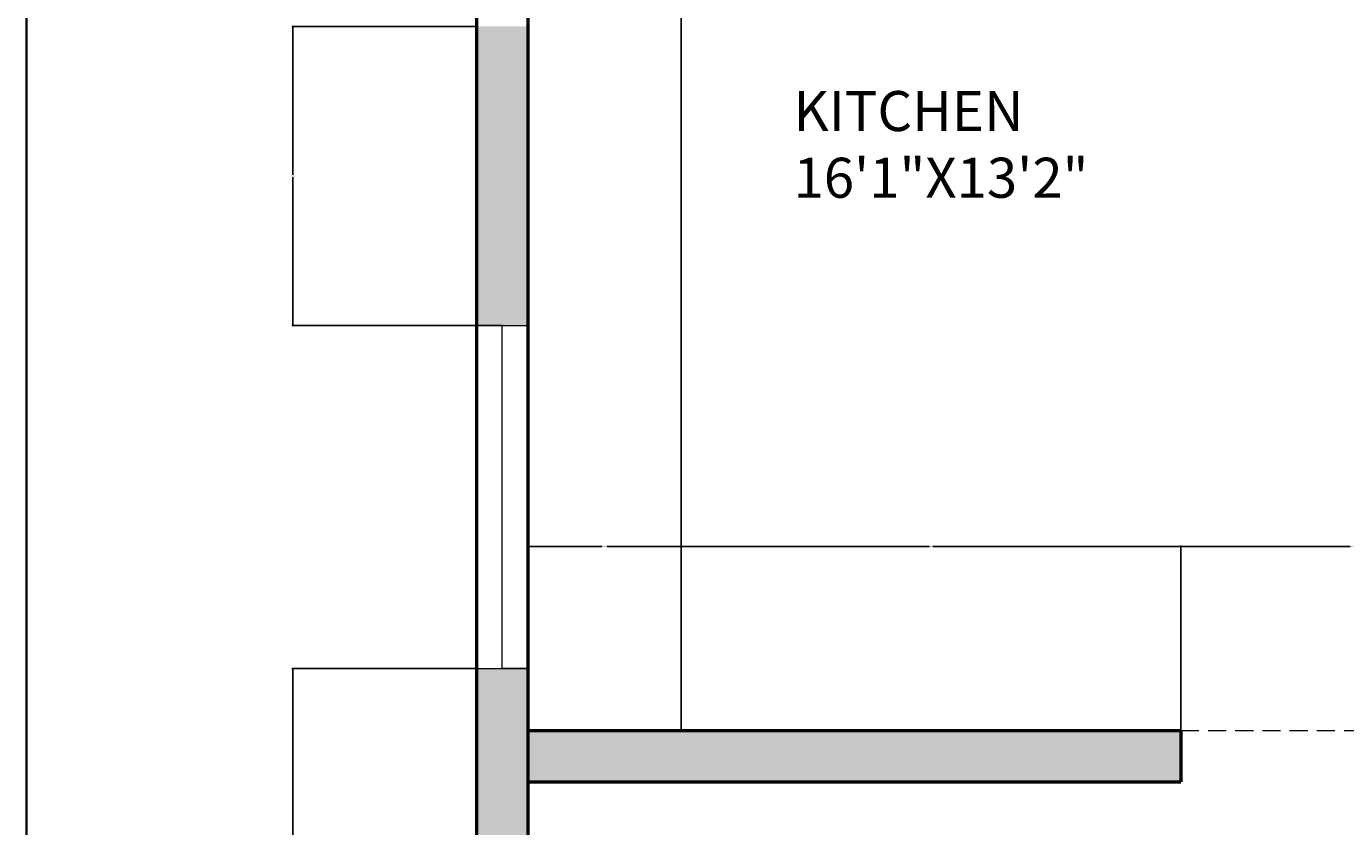
# Model space of a CAD drawing. Units: inches. Extents: x 1676 to 2199, y 1657 to 2783.
# Tile 5 of 10: x 1676 to 1907, y 2066 to 2206. Entities that reach past the tile are written whole.
import ezdxf

# ---------------------------------------------------------------- set-up
doc = ezdxf.new("R2010")
doc.units = ezdxf.units.IN
doc.linetypes.add('HIDDEN2', pattern=[4.7625, 3.175, -1.5875])
for name, color, linetype, lineweight in [('A-ANNO-DIMS', 2, 'Continuous', 18), ('A-ANNO-TTLB', 7, 'Continuous', 35), ('A-AREA-IDEN', 7, 'Continuous', 18), ('A-FLOR-CASE', 7, 'Continuous', 25), ('A-GLAZ', 4, 'Continuous', 18), ('A-WALL', 7, 'Continuous', 50), ('A-WALL-HIDN', 253, 'HIDDEN2', 18)]:
    doc.layers.add(name, color=color, linetype=linetype, lineweight=lineweight)
doc.layers.add('A-WALL-PATT', color=251, linetype='Continuous', lineweight=13, true_color=0x636466)
doc.styles.get("Standard").update_dxf_attribs({"font": 'arial.ttf'})
doc.dimstyles.get("Standard").update_dxf_attribs({"dimtxt": 0.18, "dimasz": 0.18, "dimexe": 0.18, "dimexo": 0.0625, "dimgap": 0.09, "dimtad": 0, "dimtih": 1, "dimtoh": 1, "dimdec": 4, "dimzin": 0, "dimdsep": 46, "dimtxsty": 'Standard', "dimcen": 0.09, "dimadec": 0, "dimazin": 0, "dimtfac": 1, "dimtdec": 4, "dimtofl": 0, "dimtmove": 0, "dimatfit": 3, "dimfxl": 1, "dimtolj": 1, "dimtzin": 0, "dimarcsym": 0})

# ---------------------------------------------------------------- blocks, each defined once
blk = doc.blocks.new('WIN-60')
for p, q in [((0, 0), (9, 0)), ((9, 0), (4.5, 0)), ((4.5, 0), (4.5, -60)), ((4.5, -60), (0, -60)), ((0, -60), (9, -60))]:
    blk.add_line(p, q)
blk = doc.blocks.new('*D26')
at = {"layer": 'A-ANNO-DIMS', "color": 0, "lineweight": -2, "transparency": 16777216}
for p, q in [((1755.01, 2093.92), (1722.74, 2093.92)), ((1722.92, 2093.74), (1722.92, 2056.93)), ((1722.92, 2019.75), (1722.92, 2056.56)), ((1755.01, 2019.57), (1722.74, 2019.57))]:
    blk.add_line(p, q, dxfattribs=at)
at = {"layer": 'A-ANNO-DIMS', "color": 0, "transparency": 16777216}
for points in [[(1722.89, 2093.74), (1722.95, 2093.74), (1722.92, 2093.92)], [(1722.89, 2019.75), (1722.95, 2019.75), (1722.92, 2019.57)]]:
    blk.add_solid(points, dxfattribs=at)
at = {"layer": 'Defpoints', "color": 0, "transparency": 16777216}
for p in [(1722.92, 2093.92), (1755.07, 2093.92), (1755.07, 2019.57)]:
    blk.add_point(p, dxfattribs=at)
at = {"layer": 'A-ANNO-DIMS', "color": 0, "transparency": 16777216, "insert": (1722.92, 2056.75), "char_height": 0.18, "attachment_point": 5}
blk.add_mtext('\\A1;74.35', dxfattribs=at)
blk = doc.blocks.new('*D27')
at = {"layer": 'A-ANNO-DIMS', "color": 0, "lineweight": -2, "transparency": 16777216}
for p, q in [((1755.01, 2206.26), (1722.74, 2206.26)), ((1722.92, 2206.08), (1722.92, 2180.27)), ((1722.92, 2154.1), (1722.92, 2179.91)), ((1755.01, 2153.92), (1722.74, 2153.92))]:
    blk.add_line(p, q, dxfattribs=at)
at = {"layer": 'A-ANNO-DIMS', "color": 0, "transparency": 16777216}
for points in [[(1722.89, 2206.08), (1722.95, 2206.08), (1722.92, 2206.26)], [(1722.89, 2154.1), (1722.95, 2154.1), (1722.92, 2153.92)]]:
    blk.add_solid(points, dxfattribs=at)
at = {"layer": 'Defpoints', "color": 0, "transparency": 16777216}
for p in [(1722.92, 2206.26), (1755.07, 2206.26), (1755.07, 2153.92)]:
    blk.add_point(p, dxfattribs=at)
at = {"layer": 'A-ANNO-DIMS', "color": 0, "transparency": 16777216, "insert": (1722.92, 2180.09), "char_height": 0.18, "attachment_point": 5}
blk.add_mtext('\\A1;52.34', dxfattribs=at)
blk = doc.blocks.new('*D49')
at = {"layer": 'A-ANNO-DIMS', "color": 0, "lineweight": -2, "transparency": 16777216}
for p, q in [((1878.39, 2083.15), (1878.39, 2115.42)), ((1878.57, 2115.24), (1908.02, 2115.24)), ((1938.22, 2115.24), (1908.78, 2115.24)), ((1938.4, 2083.15), (1938.4, 2115.42))]:
    blk.add_line(p, q, dxfattribs=at)
at = {"layer": 'A-ANNO-DIMS', "color": 0, "transparency": 16777216}
for points in [[(1878.57, 2115.27), (1878.57, 2115.21), (1878.39, 2115.24)], [(1938.22, 2115.27), (1938.22, 2115.21), (1938.4, 2115.24)]]:
    blk.add_solid(points, dxfattribs=at)
at = {"layer": 'Defpoints', "color": 0, "transparency": 16777216}
for p in [(1938.4, 2115.24), (1878.39, 2083.09), (1938.4, 2083.09)]:
    blk.add_point(p, dxfattribs=at)
at = {"layer": 'A-ANNO-DIMS', "color": 0, "transparency": 16777216, "insert": (1908.4, 2115.24), "char_height": 0.18, "attachment_point": 5}
blk.add_mtext('\\A1;60.01', dxfattribs=at)
blk = doc.blocks.new('*D50')
at = {"layer": 'A-ANNO-DIMS', "color": 0, "lineweight": -2, "transparency": 16777216}
for p, q in [((1790.9, 2083.15), (1790.9, 2115.42)), ((1791.08, 2115.24), (1834.32, 2115.24)), ((1878.21, 2115.24), (1834.97, 2115.24)), ((1878.39, 2083.15), (1878.39, 2115.42))]:
    blk.add_line(p, q, dxfattribs=at)
at = {"layer": 'A-ANNO-DIMS', "color": 0, "transparency": 16777216}
for points in [[(1791.08, 2115.27), (1791.08, 2115.21), (1790.9, 2115.24)], [(1878.21, 2115.27), (1878.21, 2115.21), (1878.39, 2115.24)]]:
    blk.add_solid(points, dxfattribs=at)
at = {"layer": 'Defpoints', "color": 0, "transparency": 16777216}
for p in [(1878.39, 2115.24), (1790.9, 2083.09), (1878.39, 2083.09)]:
    blk.add_point(p, dxfattribs=at)
at = {"layer": 'A-ANNO-DIMS', "color": 0, "transparency": 16777216, "insert": (1834.64, 2115.24), "char_height": 0.18, "attachment_point": 5}
blk.add_mtext('\\A1;87.5', dxfattribs=at)
blk = doc.blocks.new('*D51')
at = {"layer": 'A-ANNO-DIMS', "color": 0, "lineweight": -2, "transparency": 16777216}
for p, q in [((1764.07, 2083.15), (1764.07, 2115.42)), ((1764.25, 2115.24), (1777.09, 2115.24)), ((1790.72, 2115.24), (1777.88, 2115.24)), ((1790.9, 2083.15), (1790.9, 2115.42))]:
    blk.add_line(p, q, dxfattribs=at)
at = {"layer": 'A-ANNO-DIMS', "color": 0, "transparency": 16777216}
for points in [[(1764.25, 2115.27), (1764.25, 2115.21), (1764.07, 2115.24)], [(1790.72, 2115.27), (1790.72, 2115.21), (1790.9, 2115.24)]]:
    blk.add_solid(points, dxfattribs=at)
at = {"layer": 'Defpoints', "color": 0, "transparency": 16777216}
for p in [(1790.9, 2115.24), (1764.07, 2083.09), (1790.9, 2083.09)]:
    blk.add_point(p, dxfattribs=at)
at = {"layer": 'A-ANNO-DIMS', "color": 0, "transparency": 16777216, "insert": (1777.49, 2115.24), "char_height": 0.18, "attachment_point": 5}
blk.add_mtext('\\A1;26.82', dxfattribs=at)

msp = doc.modelspace()

# ---------------------------------------------------------------- hatches: boundary and pattern name
at = {"layer": 'A-WALL-PATT'}
h = msp.add_hatch(color=256, dxfattribs=at)
h.dxf.hatch_style = 1
h.paths.add_polyline_path([(1945.4216, 2336.5871), (1945.4216, 2341.0871), (1755.075, 2341.0871), (1755.075, 2323.0739), (1764.075, 2323.0739), (1764.075, 2332.0871), (1945.4216, 2332.0871)])
h.paths.add_polyline_path([(1764.075, 2299.0739), (1755.075, 2299.0739), (1755.075, 2266.2601), (1759.575, 2266.2601), (1764.075, 2266.2601)])
h.paths.add_polyline_path([(1843.075, 2285.0871), (1764.075, 2285.0871), (1764.075, 2276.0871), (1843.075, 2276.0871)])
h.paths.add_polyline_path([(1931.075, 2332.0871), (1922.075, 2332.0871), (1922.075, 2285.0871), (1907.247, 2285.0871), (1907.247, 2276.0871), (1922.075, 2276.0871), (1922.075, 2263.0871), (1922.075, 2214.434), (1922.075, 2183.2198), (1931.075, 2183.2198), (1931.075, 2214.434), (1931.075, 2227.0871), (1991.075, 2227.0871), (1991.075, 2176.0871), (1991.075, 2167.0871), (2000.075, 2167.0871), (2133.075, 2167.0871), (2133.075, 2176.0871), (2000.075, 2176.0871), (2000.075, 2245.3418), (1995.575, 2245.3418), (1991.075, 2245.3418), (1991.075, 2236.0871), (1931.075, 2236.0871)])
h.paths.add_polyline_path([(2000.075, 2332.0871), (1991.075, 2332.0871), (1991.075, 2285.0871), (1991.075, 2274.6339), (2000.075, 2274.6339), (2000.075, 2285.0871)], flags=17)
h.paths.add_polyline_path([(2142.075, 2341.0871), (1969.4216, 2341.0871), (1969.4216, 2332.0871), (2133.075, 2332.0871), (2133.075, 2298.2101), (2142.075, 2298.2101)])
h.paths.add_polyline_path([(2142.075, 1844.9908), (2133.075, 1844.9908), (2133.075, 1790.0871), (2061.2106, 1790.0871), (2061.2106, 1781.0871), (2142.075, 1781.0871)])
h.paths.add_polyline_path([(2001.2106, 1790.0871), (1966.075, 1790.0871), (1966.075, 1957.0871), (1973.4183, 1957.0871), (1973.4183, 1966.0871), (1966.075, 1966.0871), (1966.075, 1983.1515), (1957.075, 1983.1515), (1957.075, 1899.0871), (1946.8789, 1899.0871), (1946.8789, 1890.0871), (1957.075, 1890.0871), (1957.075, 1781.0871), (2001.2106, 1781.0871), (2001.2106, 1785.5871)])
h.paths.add_polyline_path([(1876.3163, 1894.5871), (1876.3163, 1899.0871), (1820.9237, 1899.0871), (1820.9237, 1890.0871), (1876.3163, 1890.0871)])
h.paths.add_polyline_path([(1764.075, 2093.9207), (1759.575, 2093.9207), (1755.075, 2093.9207), (1755.075, 2019.5723), (1764.075, 2019.5723)])
h.paths.add_polyline_path([(1878.3926, 2083.0871), (1764.075, 2083.0871), (1764.075, 2074.0871), (1878.3926, 2074.0871)])
h.paths.add_polyline_path([(1764.075, 1959.5723), (1755.075, 1959.5723), (1755.075, 1890.0871), (1784.9237, 1890.0871), (1784.9237, 1894.5871), (1784.9237, 1899.0871), (1764.075, 1899.0871)])
h.paths.add_polyline_path([(2133.075, 2047.0871), (2000.075, 2047.0871), (1966.075, 2047.0871), (1957.075, 2047.0871), (1938.4046, 2047.0871), (1938.4046, 2038.0871), (1957.075, 2038.0871), (1957.075, 2026.1604), (1966.075, 2026.1604), (1966.075, 2038.0871), (2039.075, 2038.0871), (2039.075, 2011.4216), (2048.075, 2011.4216), (2048.075, 2038.0871), (2133.075, 2038.0871)])
h.paths.add_polyline_path([(2133.075, 1966.0871), (2048.075, 1966.0871), (2048.075, 1972.5045), (2039.075, 1972.5045), (2039.075, 1966.0871), (2025.1075, 1966.0871), (2025.1075, 1957.0871), (2133.075, 1957.0871)])
h.paths.add_polyline_path([(1764.075, 2206.2601), (1755.075, 2206.2601), (1755.075, 2153.9207), (1764.075, 2153.9207)])

# ---------------------------------------------------------------- linework, layer by layer
at = {"layer": 'A-ANNO-TTLB'}
msp.add_lwpolyline([(1676.2722, 2782.5054), (2199.4461, 2782.5054), (2199.4461, 1657.2705), (1676.2722, 1657.2705)], close=True, dxfattribs=at)
at = {"layer": 'A-FLOR-CASE'}
msp.add_line((1790.8966, 2247.5974), (1790.8966, 2083.0871), dxfattribs=at)
at = {"layer": 'A-WALL'}
for p, q in [((1755.075, 2341.0871), (1755.075, 1890.0871)), ((1764.075, 2332.0871), (1764.075, 1899.0871)), ((1764.075, 2083.0871), (1878.3926, 2083.0871)), ((1878.3926, 2083.0871), (1878.3926, 2074.0871)), ((1764.075, 2074.0871), (1878.3926, 2074.0871))]:
    msp.add_line(p, q, dxfattribs=at)
at = {"layer": 'A-WALL-HIDN'}
msp.add_line((1878.3926, 2083.0871), (1938.4046, 2083.0871), dxfattribs=at)

# ---------------------------------------------------------------- block references
at = {"layer": 'A-GLAZ', "extrusion": (0, 0, -1), "zscale": -1, "rotation": 180}
msp.add_blockref('WIN-60', (-1755.075, 2093.9207), dxfattribs=at)

# ---------------------------------------------------------------- texts
at = {"layer": 'A-AREA-IDEN', "insert": (1810.5871, 2194.9521), "char_height": 7, "attachment_point": 1}
msp.add_mtext_dynamic_manual_height_columns('KITCHEN\\P16\'1"X13\'2"', width=180.487833, gutter_width=12.5, heights=[0], dxfattribs=at)

# ---------------------------------------------------------------- dimensions: what is measured, and where the dimension line sits
at = {"layer": 'A-ANNO-DIMS'}
for base, p1, p2, picture, middle in [((1722.925, 2206.2601), (1755.075, 2153.9207), (1755.075, 2206.2601), '*D27', (1722.925, 2180.0904)), ((1722.925, 2093.9207), (1755.075, 2019.5723), (1755.075, 2093.9207), '*D26', (1722.925, 2056.7465))]:
    dim = msp.add_linear_dim(base=base, p1=p1, p2=p2, angle=90, dimstyle='Standard', override={"dimdec": 2, "dimlfac": 1, "dimrnd": 0, "dimzin": 0, "dimdsep": 46, "dimlunit": 2}, dxfattribs=at)
    dim.commit()
    dim.dimension.update_dxf_attribs({"geometry": picture, "text_midpoint": middle})
for base, p1, p2, override, picture, middle in [((1790.8966, 2115.2371), (1764.075, 2083.0871), (1790.8966, 2083.0871), {"dimdec": 2, "dimlfac": 1, "dimrnd": 0, "dimzin": 0, "dimdsep": 46, "dimlunit": 2}, '*D51', (1777.4858, 2115.2371)), ((1878.3926, 2115.2371), (1790.8966, 2083.0871), (1878.3926, 2083.0871), {"dimdec": 1, "dimlfac": 1, "dimrnd": 0, "dimzin": 0, "dimdsep": 46, "dimlunit": 2}, '*D50', (1834.6446, 2115.2371)), ((1938.4046, 2115.2371), (1878.3926, 2083.0871), (1938.4046, 2083.0871), {"dimdec": 2, "dimlfac": 1, "dimrnd": 0, "dimzin": 0, "dimdsep": 46, "dimlunit": 2}, '*D49', (1908.3986, 2115.2371))]:
    dim = msp.add_linear_dim(base=base, p1=p1, p2=p2, dimstyle='Standard', override=override, dxfattribs=at)
    dim.commit()
    dim.dimension.update_dxf_attribs({"geometry": picture, "text_midpoint": middle})

doc.saveas('drawing.dxf')
